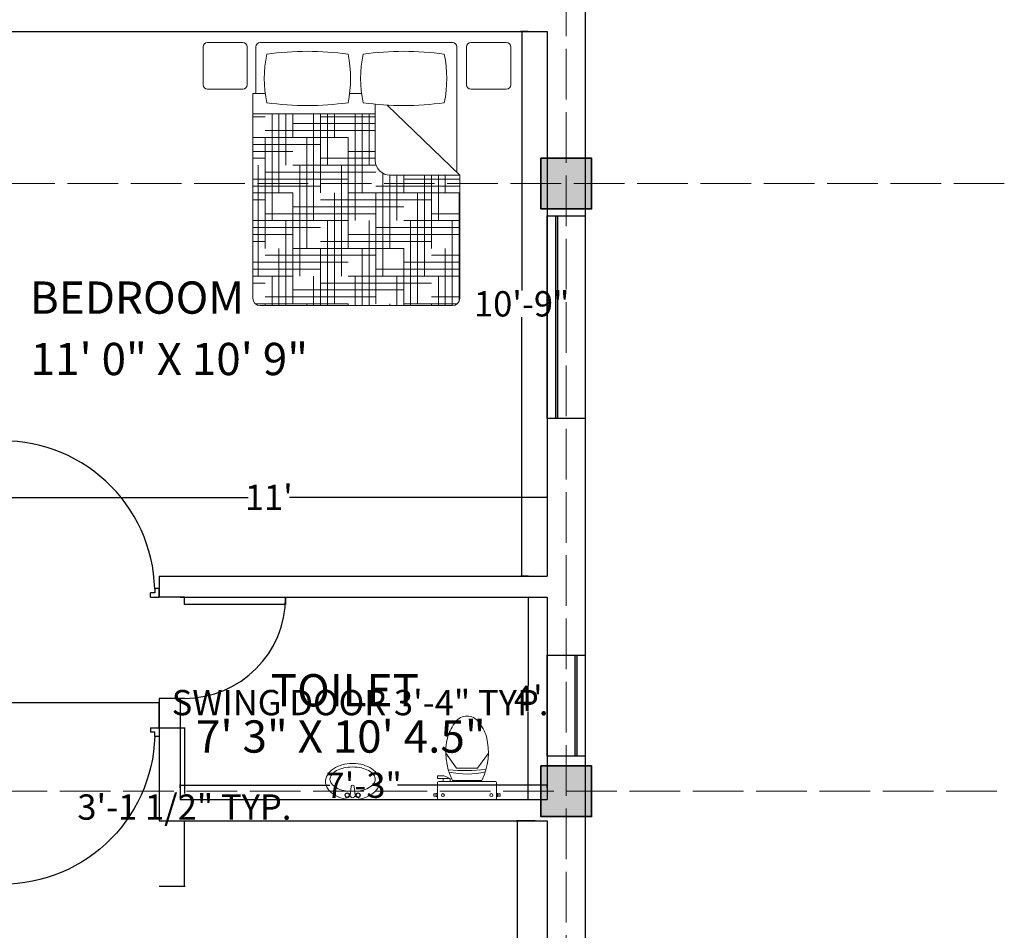
# Model space of a CAD drawing. Units: inches. Extents: x -113 to 5399, y -1393 to 3302.
# Tile 35 of 40: x 3530 to 3763, y 2688 to 2903. Entities that reach past the tile are written whole.
import ezdxf

# ---------------------------------------------------------------- set-up
doc = ezdxf.new("R2010")
doc.units = ezdxf.units.IN
doc.header["$MEASUREMENT"] = 0
doc.linetypes.add('ACAD_ISO02W100', pattern=[15, 12, -3])
for name, color, linetype, lineweight in [('A-ANNO-DIMS', 254, 'Continuous', 18), ('A-AREA-IDEN', 4, 'Continuous', 18), ('A-COLS', 7, 'Continuous', 35), ('A-FLOR-FIXT', 8, 'Continuous', 18), ('doors', 2, 'Continuous', 25), ('furniture', 131, 'Continuous', 18), ('GRIDS', 7, 'ACAD_ISO02W100', 13), ('walls', 1, 'Continuous', 25), ('windows', 3, 'Continuous', 25)]:
    doc.layers.add(name, color=color, linetype=linetype, lineweight=lineweight)
doc.styles.get("Standard").update_dxf_attribs({"font": 'arial.ttf'})
doc.dimstyles.get("Standard").update_dxf_attribs({"dimtxt": 6, "dimasz": 0.18, "dimexe": 0.18, "dimexo": 0.0625, "dimgap": 0.09, "dimtad": 0, "dimtih": 1, "dimtoh": 1, "dimdec": 1, "dimzin": 0, "dimdsep": 46, "dimlunit": 4, "dimtxsty": 'Standard', "dimblk": 'ARCHTICK', "dimcen": 0.09, "dimadec": 0, "dimazin": 0, "dimtfac": 1, "dimtdec": 1, "dimtofl": 0, "dimtmove": 0, "dimatfit": 3, "dimfxl": 1, "dimtolj": 1, "dimtzin": 0, "dimarcsym": 0})

# ---------------------------------------------------------------- blocks, each defined once
blk = doc.blocks.new('*U2')
for p, q in [((0, 0), (0, -6)), ((24, 0), (24, -6))]:
    blk.add_line(p, q)
blk.add_lwpolyline([(0, 0), (0, 24), (1.75, 24), (1.75, 0)], close=True)
blk.add_arc((0, 0), 24, 0, 90)
blk = doc.blocks.new('*X4')
at = {"color": 0}
for p, q in [((4.3594, 18.5625), (4.3594, 18.6457)), ((4.5, 18), (4.5, 18.6457)), ((4.5469, 18.1875), (4.5469, 18.6457)), ((4.5938, 18.375), (4.5938, 18.6457)), ((4.6406, 18.5625), (4.6406, 18.6457)), ((4.6875, 18.6094), (5.4375, 18.6094)), ((4.7812, 18), (4.7812, 18.6457)), ((4.8281, 18.1875), (4.8281, 18.6457)), ((4.875, 18.375), (4.875, 18.6457)), ((4.9219, 18.5625), (4.9219, 18.6457)), ((5.0625, 18), (5.0625, 18.6457)), ((5.1094, 18.1875), (5.1094, 18.6457)), ((5.1562, 18.375), (5.1562, 18.6457)), ((5.2031, 18.5625), (5.2031, 18.6457)), ((5.3438, 18), (5.3438, 18.6457)), ((5.3906, 18.1875), (5.3906, 18.6457)), ((5.4375, 18.375), (5.4375, 18.6457)), ((5.4844, 18.5625), (5.4844, 18.6457)), ((5.625, 18), (5.625, 18.6287)), ((4.4531, 17.8169), (4.4531, 18.5625)), ((4.5, 18.5625), (5.25, 18.5625)), ((4.7344, 17.8125), (4.7344, 18.5625)), ((5.0156, 17.8125), (5.0156, 18.5625)), ((5.2969, 17.8125), (5.2969, 18.5625)), ((5.5781, 17.8125), (5.5781, 18.5625)), ((5.625, 18.5625), (5.6375, 18.5625)), ((4.3395, 18.5156), (5.0625, 18.5156)), ((4.3395, 18.4688), (4.875, 18.4688)), ((5.25, 18.4688), (5.6375, 18.4688)), ((5.4375, 18.5156), (5.6375, 18.5156)), ((4.3395, 18.4219), (4.6875, 18.4219)), ((5.0625, 18.4219), (5.6375, 18.4219)), ((4.3395, 18.375), (4.5, 18.375)), ((4.4062, 17.8169), (4.4062, 18.375)), ((4.6875, 17.8114), (4.6875, 18.375)), ((4.6875, 18.3281), (5.4375, 18.3281)), ((4.875, 18.375), (5.625, 18.375)), ((4.9688, 17.625), (4.9688, 18.375)), ((5.25, 17.625), (5.25, 18.375)), ((5.5312, 17.625), (5.5312, 18.375)), ((4.5, 18.2812), (5.25, 18.2812)), ((5.625, 18.2812), (5.6375, 18.2812)), ((4.3395, 18.2344), (5.0625, 18.2344)), ((5.4375, 18.2344), (5.6375, 18.2344)), ((4.3395, 18.1875), (4.875, 18.1875)), ((4.3395, 18.1406), (4.6875, 18.1406)), ((4.3594, 17.8169), (4.3594, 18.1875)), ((4.6406, 17.8169), (4.6406, 18.1875)), ((4.9219, 17.4375), (4.9219, 18.1875)), ((5.0625, 18.1406), (5.6375, 18.1406)), ((5.2031, 17.4375), (5.2031, 18.1875)), ((5.25, 18.1875), (5.6375, 18.1875)), ((5.4844, 17.4375), (5.4844, 18.1875)), ((4.3395, 18.0938), (4.5, 18.0938)), ((4.875, 18.0938), (5.625, 18.0938)), ((4.5, 18), (5.25, 18)), ((4.5938, 17.8169), (4.5938, 18)), ((4.6875, 18.0469), (5.4375, 18.0469)), ((4.875, 17.25), (4.875, 18)), ((5.1562, 17.25), (5.1562, 18)), ((5.4375, 17.25), (5.4375, 18)), ((5.625, 18), (5.6375, 18)), ((4.3395, 17.9531), (5.0625, 17.9531)), ((5.4375, 17.9531), (5.6375, 17.9531)), ((4.3395, 17.9062), (4.875, 17.9062)), ((4.3395, 17.8594), (4.6875, 17.8594)), ((5.0625, 17.8594), (5.6375, 17.8594)), ((5.25, 17.9062), (5.6375, 17.9062)), ((4.8281, 17.2457), (4.8281, 17.8125)), ((4.875, 17.8125), (5.625, 17.8125)), ((5.1094, 17.2457), (5.1094, 17.8125)), ((5.3906, 17.2457), (5.3906, 17.8125)), ((4.7421, 17.7656), (5.4375, 17.7656)), ((4.7548, 17.7188), (5.25, 17.7188)), ((4.7548, 17.6719), (5.0625, 17.6719)), ((5.4375, 17.6719), (5.6375, 17.6719)), ((5.625, 17.7188), (5.6375, 17.7188)), ((4.7548, 17.625), (4.875, 17.625)), ((4.7812, 17.2457), (4.7812, 17.625)), ((5.0625, 17.2457), (5.0625, 17.625)), ((5.25, 17.625), (5.6375, 17.625)), ((5.3438, 17.2457), (5.3438, 17.625)), ((5.625, 17.2627), (5.625, 17.625)), ((4.875, 17.5312), (5.625, 17.5312)), ((5.0625, 17.5781), (5.6375, 17.5781)), ((4.7548, 17.4844), (5.4375, 17.4844)), ((4.7548, 17.4375), (5.25, 17.4375)), ((4.7548, 17.3906), (5.0625, 17.3906)), ((5.0156, 17.2457), (5.0156, 17.4375)), ((5.2969, 17.2457), (5.2969, 17.4375)), ((5.4375, 17.3906), (5.6375, 17.3906)), ((5.5781, 17.2457), (5.5781, 17.4375)), ((5.625, 17.4375), (5.6375, 17.4375)), ((4.7548, 17.3438), (4.875, 17.3438)), ((5.25, 17.3438), (5.6375, 17.3438)), ((5.0625, 17.2969), (5.6375, 17.2969)), ((4.875, 17.25), (5.6077, 17.25)), ((4.9688, 17.2457), (4.9688, 17.25)), ((5.25, 17.2457), (5.25, 17.25)), ((5.5312, 17.2457), (5.5312, 17.25))]:
    blk.add_line(p, q, dxfattribs=at)
blk = doc.blocks.new('MAT-P01')
for p, q in [((-0.0213, 0.8164), (-0.0213, 0.5605)), ((0.0087, 0.8464), (0.2471, 0.8464)), ((0.2771, 0.8164), (0.2771, 0.5605)), ((0.3437, 0.8164), (0.3437, -0.0316)), ((0.3737, 0.8464), (1.6737, 0.8464)), ((1.7037, 0.8164), (1.7037, 0.5005)), ((1.7622, 0.8164), (1.7622, 0.5605)), ((1.7922, 0.8464), (2.0306, 0.8464)), ((2.0606, 0.8164), (2.0606, 0.5605)), ((0.0087, 0.5305), (0.2471, 0.5305)), ((0.9879, 0.5005), (1.0693, 0.5005)), ((1.6393, 0.5005), (1.7237, 0.5005)), ((1.7237, 0.5005), (1.7237, -0.8836)), ((1.7922, 0.5305), (2.0306, 0.5305)), ((0.8146, 0.423), (0.3237, -0.0509)), ((0.8949, 0.4293), (0.8949, 0.0491)), ((0.8949, 0.3643), (1.7237, 0.3643)), ((0.8949, 0.3643), (0.8949, 0.0491)), ((0.8949, 0.3643), (1.7237, 0.3643)), ((1.7237, 0.3643), (1.7237, -0.8836)), ((0.3237, -0.0509), (0.7949, -0.0509)), ((0.3237, -0.0509), (0.3237, -0.8836)), ((0.3737, -0.9336), (1.6737, -0.9336))]:
    blk.add_line(p, q)
for centre, radius, start, end in [((0.0087, 0.8164), 0.03, 90, 180), ((0.2471, 0.8164), 0.03, 0, 90), ((0.3737, 0.8164), 0.03, 90, 180), ((1.6737, 0.8164), 0.03, 0, 90), ((1.7922, 0.8164), 0.03, 90, 180), ((2.0306, 0.8164), 0.03, 0, 90), ((1.2251, 0.6034), 0.8138, 168.37298, 191.62702), ((0.7029, -1.1436), 1.9306, 81.81622, 98.18378), ((0.1806, 0.6034), 0.8138, 348.37298, 11.62702), ((1.8766, 0.6034), 0.8138, 168.37298, 191.62702), ((1.3543, -1.1436), 1.9306, 81.81622, 98.18378), ((0.8321, 0.6034), 0.8138, 348.37298, 11.62702), ((0.0087, 0.5605), 0.03, 180, 270), ((0.2471, 0.5605), 0.03, 270, 0), ((1.7922, 0.5605), 0.03, 180, 270), ((2.0306, 0.5605), 0.03, 270, 0), ((0.7029, 2.3504), 1.9306, 261.81622, 278.18378), ((1.3543, 2.3504), 1.9306, 261.81622, 278.18378), ((0.7949, 0.0491), 0.1, 270, 0), ((0.3737, -0.8836), 0.05, 180, 270), ((1.6737, -0.8836), 0.05, 270, 0)]:
    blk.add_arc(centre, radius, start, end)
at = {"rotation": 270}
blk.add_blockref('*X4', (-16.9221, 4.7038), dxfattribs=at)
blk = doc.blocks.new('toilet-3')
at = {"color": 0, "linetype": 'ByBlock'}
for p, q in [((-0.2813, -0.0495), (-0.2813, -0.069)), ((-0.2813, -0.0495), (-0.2613, -0.0495)), ((-0.2813, -0.069), (-0.2613, -0.069)), ((-0.2613, -0.0467), (-0.2613, -0.0717)), ((-0.2613, -0.0467), (-0.2513, -0.0467)), ((-0.2613, -0.0717), (-0.2513, -0.0717)), ((-0.2513, -0.0467), (-0.2513, -0.0717)), ((-0.25, -0.03), (-0.25, -0.1645)), ((0.24, -0.02), (-0.24, -0.02)), ((0.25, -0.03), (0.25, -0.1645)), ((0.2613, -0.0467), (0.2513, -0.0467)), ((0.2513, -0.0467), (0.2513, -0.0717)), ((0.2613, -0.0717), (0.2513, -0.0717)), ((0.2613, -0.0467), (0.2613, -0.0717)), ((0.2813, -0.0495), (0.2613, -0.0495)), ((0.2813, -0.069), (0.2613, -0.069)), ((0.2813, -0.0495), (0.2813, -0.069)), ((-0.1435, -0.1995), (-0.25, -0.1995)), ((-0.25, -0.1995), (-0.25, -0.2221)), ((-0.1981, -0.2221), (-0.25, -0.2221)), ((0.24, -0.1745), (-0.24, -0.1745)), ((-0.2025, -0.1995), (-0.2025, -0.1745)), ((-0.1981, -0.2221), (-0.1601, -0.2072)), ((-0.1601, -0.2072), (-0.1601, -0.1995)), ((-0.1435, -0.1995), (-0.1435, -0.1745)), ((0.125, -0.1821), (-0.125, -0.1821)), ((-0.0886, -0.2874), (-0.1803, -0.4145)), ((0.0886, -0.2874), (-0.0886, -0.2874)), ((0.0886, -0.2874), (0.1803, -0.4145))]:
    blk.add_line(p, q, dxfattribs=at)
for centre in [(-0.2052, -0.0592), (0.2052, -0.0592)]:
    blk.add_circle(centre, 0.0125, dxfattribs=at)
for centre, radius, start, end in [((-0.24, -0.03), 0.01, 90, 180), ((0.24, -0.03), 0.01, 0, 90), ((-0.24, -0.1645), 0.01, 180, 270), ((0.24, -0.1645), 0.01, 270, 0), ((0.3763, -0.4241), 0.5567, 154.23211, 193.67546), ((-0.0054, -0.8958), 0.6585, 75.92762, 103.02045), ((-0.3763, -0.4241), 0.5567, 346.32454, 25.76789), ((-0.013, -1.7868), 1.5207, 83.45525, 95.52712), ((0.2621, -0.4063), 0.4521, 199.29417, 217.25487), ((-0.265, -0.4003), 0.4568, 322.23824, 340.10511), ((-0.0008, -0.6086), 0.1204, 216.37945, 323.62055)]:
    blk.add_arc(centre, radius, start, end, dxfattribs=at)
blk = doc.blocks.new('wash-6')
at = {"color": 0, "linetype": 'ByBlock'}
for p, q in [((-0.036, -0.063), (-0.021, -0.18)), ((0.036, -0.063), (0.021, -0.18))]:
    blk.add_line(p, q, dxfattribs=at)
for centre, radius in [((-0.075, -0.062), 0.0325), ((-0.075, -0.062), 0.0263), ((0.075, -0.062), 0.0325), ((0.075, -0.062), 0.0263)]:
    blk.add_circle(centre, radius, dxfattribs=at)
for centre, radius, start, end in [((0, -0.56), 0.56, 90, 105.4371), ((-0.107, -0.311), 0.285, 123.6901, 148.1465), ((-0.042, -0.407), 0.401, 105.4371, 123.6901), ((-0.045, -0.488), 0.37, 102.6081, 118.369), ((0, -0.69), 0.576, 92.9466, 102.6081), ((0, -0.063), 0.0361, 0, 180), ((0, -0.56), 0.56, 74.5629, 90), ((0, -0.69), 0.576, 77.3919, 87.0534), ((0.045, -0.488), 0.37, 61.631, 77.3919), ((0.042, -0.407), 0.401, 56.3099, 74.5629), ((0.107, -0.311), 0.285, 31.8535, 56.3099), ((-0.204, -0.25), 0.17, 148.1465, 180), ((-0.204, -0.25), 0.17, 180, 211.8535), ((-0.217, -0.282), 0.0954, 142.5096, 180), ((-0.114, -0.361), 0.225, 118.369, 142.5096), ((0, -0.18), 0.0215, 180, 0), ((0.114, -0.361), 0.225, 37.4904, 61.631), ((0.217, -0.282), 0.0954, 0, 37.4904), ((0.204, -0.25), 0.17, 0, 31.8535), ((0.204, -0.25), 0.17, 328.1465, 0), ((-0.107, -0.189), 0.285, 211.8535, 236.3099), ((-0.217, -0.282), 0.0954, 180, 217.4904), ((-0.114, -0.203), 0.225, 217.4904, 241.631), ((-0.045, -0.076), 0.37, 241.631, 257.3919), ((0.045, -0.076), 0.37, 282.6081, 298.369), ((0.114, -0.203), 0.225, 298.369, 322.5096), ((0.107, -0.189), 0.285, 303.6901, 328.1465), ((0.217, -0.282), 0.0954, 322.5096, 0), ((-0.042, -0.092), 0.401, 236.3099, 254.5629), ((0, 0.06), 0.56, 254.5629, 270), ((0, 0.125), 0.576, 257.3919, 270), ((0, 0.125), 0.576, 270, 282.6081), ((0, 0.06), 0.56, 270, 285.4371), ((0.042, -0.092), 0.401, 285.4371, 303.6901)]:
    blk.add_arc(centre, radius, start, end, dxfattribs=at)
blk = doc.blocks.new('_ArchTick')
at = {"color": 0, "linetype": 'ByBlock', "const_width": 0.15}
blk.add_lwpolyline([(-0.5, -0.5), (0.5, 0.5)], dxfattribs=at)
blk = doc.blocks.new('*D141')
at = {"layer": 'A-ANNO-DIMS', "color": 0, "lineweight": -2, "transparency": 16777216}
for p, q in [((3651.65, 2713.56), (3647.23, 2713.56)), ((3647.41, 2713.56), (3647.41, 2658.47)), ((3647.41, 2589.06), (3647.41, 2644.14)), ((3651.65, 2589.06), (3647.23, 2589.06))]:
    blk.add_line(p, q, dxfattribs=at)
at = {"layer": 'Defpoints', "color": 0, "transparency": 16777216}
for p in [(3651.72, 2713.56), (3647.41, 2589.06), (3651.72, 2589.06)]:
    blk.add_point(p, dxfattribs=at)
at = {"layer": 'A-ANNO-DIMS', "color": 0, "lineweight": -2, "transparency": 16777216, "xscale": 0.18, "yscale": 0.18, "zscale": 0.18}
for p, rotation in [((3647.41, 2713.56), 90), ((3647.41, 2589.06), 270)]:
    blk.add_blockref('_ArchTick', p, dxfattribs=dict(at, rotation=rotation))
at = {"layer": 'A-ANNO-DIMS', "color": 0, "transparency": 16777216, "insert": (3647.41, 2651.31), "char_height": 6, "attachment_point": 5}
blk.add_mtext('\\A1;10\'-4{\\H1x;\\S1/2;}"', dxfattribs=at)
blk = doc.blocks.new('*D144')
at = {"layer": 'A-ANNO-DIMS', "color": 0, "lineweight": -2, "transparency": 16777216}
for p, q in [((3650.05, 2766.56), (3650.05, 2745.65)), ((3650.06, 2766.56), (3650.23, 2766.56)), ((3650.05, 2718.56), (3650.05, 2739.47)), ((3650.06, 2718.56), (3650.23, 2718.56))]:
    blk.add_line(p, q, dxfattribs=at)
at = {"layer": 'Defpoints', "color": 0, "transparency": 16777216}
for p in [(3650, 2766.56), (3650, 2718.56), (3650.05, 2718.56)]:
    blk.add_point(p, dxfattribs=at)
at = {"layer": 'A-ANNO-DIMS', "color": 0, "lineweight": -2, "transparency": 16777216, "xscale": 0.18, "yscale": 0.18, "zscale": 0.18}
for p, rotation in [((3650.05, 2766.56), 90), ((3650.05, 2718.56), 270)]:
    blk.add_blockref('_ArchTick', p, dxfattribs=dict(at, rotation=rotation))
at = {"layer": 'A-ANNO-DIMS', "color": 0, "transparency": 16777216, "insert": (3650.05, 2742.56), "char_height": 6, "attachment_point": 5}
blk.add_mtext("\\A1;4'", dxfattribs=at)
blk = doc.blocks.new('*D145')
at = {"layer": 'A-ANNO-DIMS', "color": 0, "lineweight": -2, "transparency": 16777216}
for p, q in [((3567.55, 2721.36), (3567.55, 2722.17)), ((3567.55, 2721.99), (3603.01, 2721.99)), ((3654.55, 2721.99), (3619.09, 2721.99)), ((3654.55, 2721.36), (3654.55, 2722.17))]:
    blk.add_line(p, q, dxfattribs=at)
at = {"layer": 'Defpoints', "color": 0, "transparency": 16777216}
for p in [(3567.55, 2721.99), (3567.55, 2721.3), (3654.55, 2721.3)]:
    blk.add_point(p, dxfattribs=at)
at = {"layer": 'A-ANNO-DIMS', "color": 0, "lineweight": -2, "transparency": 16777216, "xscale": 0.18, "yscale": 0.18, "zscale": 0.18, "rotation": 180}
blk.add_blockref('_ArchTick', (3567.55, 2721.99), dxfattribs=at)
at = {"layer": 'A-ANNO-DIMS', "color": 0, "lineweight": -2, "transparency": 16777216, "xscale": 0.18, "yscale": 0.18, "zscale": 0.18}
blk.add_blockref('_ArchTick', (3654.55, 2721.99), dxfattribs=at)
at = {"layer": 'A-ANNO-DIMS', "color": 0, "transparency": 16777216, "insert": (3611.05, 2721.99), "char_height": 6, "attachment_point": 5}
blk.add_mtext('\\A1;7\'-3"', dxfattribs=at)
blk = doc.blocks.new('*D146')
at = {"layer": 'A-ANNO-DIMS', "color": 0, "lineweight": -2, "transparency": 16777216}
for p, q in [((3650, 2900.56), (3648.31, 2900.56)), ((3648.49, 2900.56), (3648.49, 2839.21)), ((3648.49, 2771.56), (3648.49, 2832.91)), ((3650, 2771.56), (3648.31, 2771.56))]:
    blk.add_line(p, q, dxfattribs=at)
at = {"layer": 'Defpoints', "color": 0, "transparency": 16777216}
for p in [(3650.06, 2900.56), (3648.49, 2771.56), (3650.06, 2771.56)]:
    blk.add_point(p, dxfattribs=at)
at = {"layer": 'A-ANNO-DIMS', "color": 0, "lineweight": -2, "transparency": 16777216, "xscale": 0.18, "yscale": 0.18, "zscale": 0.18}
for p, rotation in [((3648.49, 2900.56), 90), ((3648.49, 2771.56), 270)]:
    blk.add_blockref('_ArchTick', p, dxfattribs=dict(at, rotation=rotation))
at = {"layer": 'A-ANNO-DIMS', "color": 0, "transparency": 16777216, "insert": (3648.49, 2836.06), "char_height": 6, "attachment_point": 5}
blk.add_mtext('\\A1;10\'-9"', dxfattribs=at)
blk = doc.blocks.new('*D147')
at = {"layer": 'A-ANNO-DIMS', "color": 0, "lineweight": -2, "transparency": 16777216}
for p, q in [((3522.55, 2790.25), (3522.55, 2790.37)), ((3522.55, 2790.19), (3583.65, 2790.19)), ((3654.55, 2790.19), (3593.45, 2790.19)), ((3654.55, 2790.25), (3654.55, 2790.37))]:
    blk.add_line(p, q, dxfattribs=at)
at = {"layer": 'Defpoints', "color": 0, "transparency": 16777216}
for p in [(3522.55, 2790.19), (3522.55, 2790.19), (3654.55, 2790.19)]:
    blk.add_point(p, dxfattribs=at)
at = {"layer": 'A-ANNO-DIMS', "color": 0, "lineweight": -2, "transparency": 16777216, "xscale": 0.18, "yscale": 0.18, "zscale": 0.18, "rotation": 180}
blk.add_blockref('_ArchTick', (3522.55, 2790.19), dxfattribs=at)
at = {"layer": 'A-ANNO-DIMS', "color": 0, "lineweight": -2, "transparency": 16777216, "xscale": 0.18, "yscale": 0.18, "zscale": 0.18}
blk.add_blockref('_ArchTick', (3654.55, 2790.19), dxfattribs=at)
at = {"layer": 'A-ANNO-DIMS', "color": 0, "transparency": 16777216, "insert": (3588.55, 2790.19), "char_height": 6, "attachment_point": 5}
blk.add_mtext("\\A1;11'", dxfattribs=at)
blk = doc.blocks.new('WIN-PLAN-48IN')
h = blk.add_hatch(color=256)
h.dxf.hatch_style = 1
h.paths.add_polyline_path([(48, 2.5), (0, 2.5), (0, 2), (48, 2)])
for p, q in [((0, 9), (48, 9)), ((0, 0), (0, 9)), ((48, 9), (48, 0)), ((48, 2.5), (0, 2.5)), ((48, 2), (0, 2)), ((48, 0), (0, 0))]:
    blk.add_line(p, q)
blk = doc.blocks.new('WIN-PLAN-24IN')
h = blk.add_hatch(color=256)
h.dxf.hatch_style = 1
h.paths.add_polyline_path([(6.5, 24), (6.5, 0), (7, 0), (7, 24)])
for p, q in [((0, 0), (0, 24)), ((0, 24), (9, 24)), ((6.5, 24), (6.5, 0)), ((7, 24), (7, 0)), ((9, 24), (9, 0)), ((9, 0), (0, 0))]:
    blk.add_line(p, q)
blk = doc.blocks.new('COLUMN-12IN-SQUARE')
h = blk.add_hatch(color=256)
h.dxf.hatch_style = 1
h.paths.add_polyline_path([(6, 6), (-6, 6), (-6, -6), (6, -6)])
blk.add_lwpolyline([(-6, 6), (6, 6), (6, -6), (-6, -6)], close=True)
blk = doc.blocks.new('DOOR-SINGLE-36IN-PLAN')
for p, q in [((0.5, 2), (0.5, 36.98)), ((0.5, 36.98), (1.5, 36.98)), ((1.5, 36.98), (1.5, 2)), ((0, 2), (0, 0)), ((0, 2), (1.04, 2)), ((1.5, 2), (0.5, 2)), ((1.04, 2), (1.04, 0.98)), ((1.04, 0.98), (2, 0.98)), ((2, 0), (2, 0.98)), ((38.96, 0.98), (38, 0.98)), ((38, 0), (38, 0.98)), ((40, 2), (38.96, 2)), ((38.96, 2), (38.96, 0.98)), ((40, 0), (40, 2)), ((0, 0), (2, 0)), ((0, 0), (2, 0)), ((38, 0), (40, 0))]:
    blk.add_line(p, q)
blk.add_arc((2.94, 0.99), 36.04, 1.6003, 93.0893)
blk = doc.blocks.new('*D175')
at = {"layer": 'A-ANNO-DIMS', "color": 0, "lineweight": -2, "transparency": 16777216}
for p, q in [((3522.55, 2735.62), (3522.55, 2741.74)), ((3562.55, 2735.62), (3562.55, 2741.74)), ((3522.55, 2741.56), (3562.55, 2741.56)), ((3562.55, 2741.56), (3562.73, 2741.56))]:
    blk.add_line(p, q, dxfattribs=at)
at = {"layer": 'Defpoints', "color": 0, "transparency": 16777216}
for p in [(3562.55, 2741.56), (3522.55, 2735.56), (3562.55, 2735.56)]:
    blk.add_point(p, dxfattribs=at)
at = {"layer": 'A-ANNO-DIMS', "color": 0, "lineweight": -2, "transparency": 16777216, "xscale": 0.18, "yscale": 0.18, "zscale": 0.18, "rotation": 180}
blk.add_blockref('_ArchTick', (3522.55, 2741.56), dxfattribs=at)
at = {"layer": 'A-ANNO-DIMS', "color": 0, "lineweight": -2, "transparency": 16777216, "xscale": 0.18, "yscale": 0.18, "zscale": 0.18}
blk.add_blockref('_ArchTick', (3562.55, 2741.56), dxfattribs=at)
at = {"layer": 'A-ANNO-DIMS', "color": 0, "transparency": 16777216, "insert": (3610.19, 2741.56), "char_height": 6, "attachment_point": 5}
blk.add_mtext('\\A1;SWING DOOR 3\'-4" TYP.', dxfattribs=at)
blk = doc.blocks.new('*D176')
at = {"layer": 'A-ANNO-DIMS', "color": 0, "lineweight": -2, "transparency": 16777216}
for p, q in [((3562.61, 2735.56), (3568.73, 2735.56)), ((3568.55, 2735.56), (3568.55, 2720)), ((3568.55, 2698.06), (3568.55, 2713.61)), ((3562.61, 2698.06), (3568.73, 2698.06))]:
    blk.add_line(p, q, dxfattribs=at)
at = {"layer": 'Defpoints', "color": 0, "transparency": 16777216}
for p in [(3562.55, 2735.56), (3562.55, 2698.06), (3568.55, 2698.06)]:
    blk.add_point(p, dxfattribs=at)
at = {"layer": 'A-ANNO-DIMS', "color": 0, "lineweight": -2, "transparency": 16777216, "xscale": 0.18, "yscale": 0.18, "zscale": 0.18}
for p, rotation in [((3568.55, 2735.56), 90), ((3568.55, 2698.06), 270)]:
    blk.add_blockref('_ArchTick', p, dxfattribs=dict(at, rotation=rotation))
at = {"layer": 'A-ANNO-DIMS', "color": 0, "transparency": 16777216, "insert": (3568.55, 2716.81), "char_height": 6, "attachment_point": 5}
blk.add_mtext('\\A1;3\'-1 1/2" TYP.', dxfattribs=at)

msp = doc.modelspace()

# ---------------------------------------------------------------- linework, layer by layer
at = {"layer": 'GRIDS'}
for p, q in [((3659.05, 3271.46), (3659.05, 2498.02)), ((3762.86, 2864.56), (3104.61, 2864.56)), ((3104.07, 2720.56), (3762.86, 2720.56))]:
    msp.add_line(p, q, dxfattribs=at)
at = {"layer": 'walls'}
for p, q in [((3663.55, 3230.06), (3663.55, 2580.06)), ((3505.55, 2900.56), (3654.55, 2900.56)), ((3654.55, 2900.56), (3654.55, 2776.06)), ((3654.55, 2776.06), (3654.55, 2771.56)), ((3562.55, 2771.56), (3562.55, 2766.56)), ((3562.55, 2771.56), (3654.55, 2771.56)), ((3567.55, 2766.56), (3562.55, 2766.56)), ((3567.55, 2766.56), (3654.55, 2766.56)), ((3654.55, 2766.56), (3654.55, 2718.56)), ((3562.55, 2742.56), (3562.55, 2713.56)), ((3567.55, 2742.56), (3562.55, 2742.56)), ((3567.55, 2742.56), (3567.55, 2718.56)), ((3567.55, 2718.56), (3654.55, 2718.56)), ((3562.55, 2713.56), (3654.55, 2713.56)), ((3654.55, 2713.56), (3654.55, 2589.06))]:
    msp.add_line(p, q, dxfattribs=at)

# ---------------------------------------------------------------- block references
at = {"layer": 'A-COLS'}
for p in [(3659.05, 2864.56), (3659.05, 2720.56)]:
    msp.add_blockref('COLUMN-12IN-SQUARE', p, dxfattribs=at)
at = {"layer": 'A-FLOR-FIXT', "rotation": 180}
for name, p, xscale, yscale, zscale in [('toilet-3', (3635.55, 2718), -27.95492935005888, 27.95492935005888, 27.95492935005888), ('wash-6', (3608.42, 2718.56), -17.16666334294967, 17.16666334294967, 17.16666334294967)]:
    msp.add_blockref(name, p, dxfattribs=dict(at, xscale=xscale, yscale=yscale, zscale=zscale))
at = {"layer": 'doors'}
msp.add_blockref('DOOR-SINGLE-36IN-PLAN', (3522.55, 2766.56), dxfattribs=at)
at = {"layer": 'doors', "rotation": 270}
msp.add_blockref('*U2', (3568.55, 2766.56), dxfattribs=at)
at = {"layer": 'doors', "extrusion": (0, 0, -1), "zscale": -1, "rotation": 180}
msp.add_blockref('DOOR-SINGLE-36IN-PLAN', (-3522.55, 2735.56), dxfattribs=at)
at = {"layer": 'furniture', "xscale": -35.02364872074636, "yscale": 35.02364872074636, "zscale": 35.02364872074636}
msp.add_blockref('MAT-P01', (3645.14, 2868.33), dxfattribs=at)
at = {"layer": 'windows', "rotation": 270.0000000000034}
msp.add_blockref('WIN-PLAN-48IN', (3654.55, 2856.92), dxfattribs=at)
at = {"layer": 'windows'}
msp.add_blockref('WIN-PLAN-24IN', (3654.55, 2728.84), dxfattribs=at)

# ---------------------------------------------------------------- texts
at = {"layer": 'A-AREA-IDEN'}
for s, height, p in [('BEDROOM', 7.647, (3531.94, 2833.71)), ('11\' 0" X 10\' 9"', 7.6473, (3532.11, 2819.16)), ('TOILET', 7.647, (3589.02, 2740.66)), ('7\' 3" X 10\' 4.5"', 7.6473, (3571.3, 2729.7))]:
    msp.add_text(s, height=height, dxfattribs=at).set_placement(p)

# ---------------------------------------------------------------- dimensions: what is measured, and where the dimension line sits
at = {"layer": 'A-ANNO-DIMS'}
for base, p1, p2, picture, middle in [((3648.49, 2771.56), (3650.06, 2900.56), (3650.06, 2771.56), '*D146', (3648.49, 2836.06)), ((3650.05, 2718.56), (3650, 2766.56), (3650, 2718.56), '*D144', (3650.05, 2742.56)), ((3647.41, 2589.06), (3651.72, 2713.56), (3651.72, 2589.06), '*D141', (3647.41, 2651.31))]:
    dim = msp.add_linear_dim(base=base, p1=p1, p2=p2, angle=90, dimstyle='Standard', override={"dimclrd": 0, "dimclre": 0, "dimclrt": 0}, dxfattribs=at)
    dim.commit()
    dim.dimension.update_dxf_attribs({"geometry": picture, "text_midpoint": middle})
for base, p1, p2, picture, middle in [((3522.55, 2790.19), (3654.55, 2790.19), (3522.55, 2790.19), '*D147', (3588.55, 2790.19)), ((3567.55, 2721.99), (3654.55, 2721.3), (3567.55, 2721.3), '*D145', (3611.05, 2721.99))]:
    dim = msp.add_linear_dim(base=base, p1=p1, p2=p2, dimstyle='Standard', override={"dimclrd": 0, "dimclre": 0, "dimclrt": 0}, dxfattribs=at)
    dim.commit()
    dim.dimension.update_dxf_attribs({"geometry": picture, "text_midpoint": middle})
dim = msp.add_linear_dim(base=(3562.55, 2741.56), p1=(3522.55, 2735.56), p2=(3562.55, 2735.56), text='SWING DOOR <> TYP.', dimstyle='Standard', override={"dimdec": 1, "dimlfac": 1, "dimrnd": 0, "dimzin": 1, "dimdsep": 46, "dimlunit": 4, "dimfrac": 2}, dxfattribs=at)
dim.commit()
dim.dimension.update_dxf_attribs({"geometry": '*D175', "text_midpoint": (3610.19, 2741.56)})
dim = msp.add_linear_dim(base=(3568.55, 2698.06), p1=(3562.55, 2735.56), p2=(3562.55, 2698.06), angle=270, text='<> TYP.', dimstyle='Standard', override={"dimdec": 1, "dimlfac": 1, "dimrnd": 0, "dimzin": 1, "dimdsep": 46, "dimlunit": 4, "dimfrac": 2}, dxfattribs=at)
dim.commit()
dim.dimension.update_dxf_attribs({"geometry": '*D176', "text_midpoint": (3568.55, 2716.81)})

doc.saveas('drawing.dxf')
